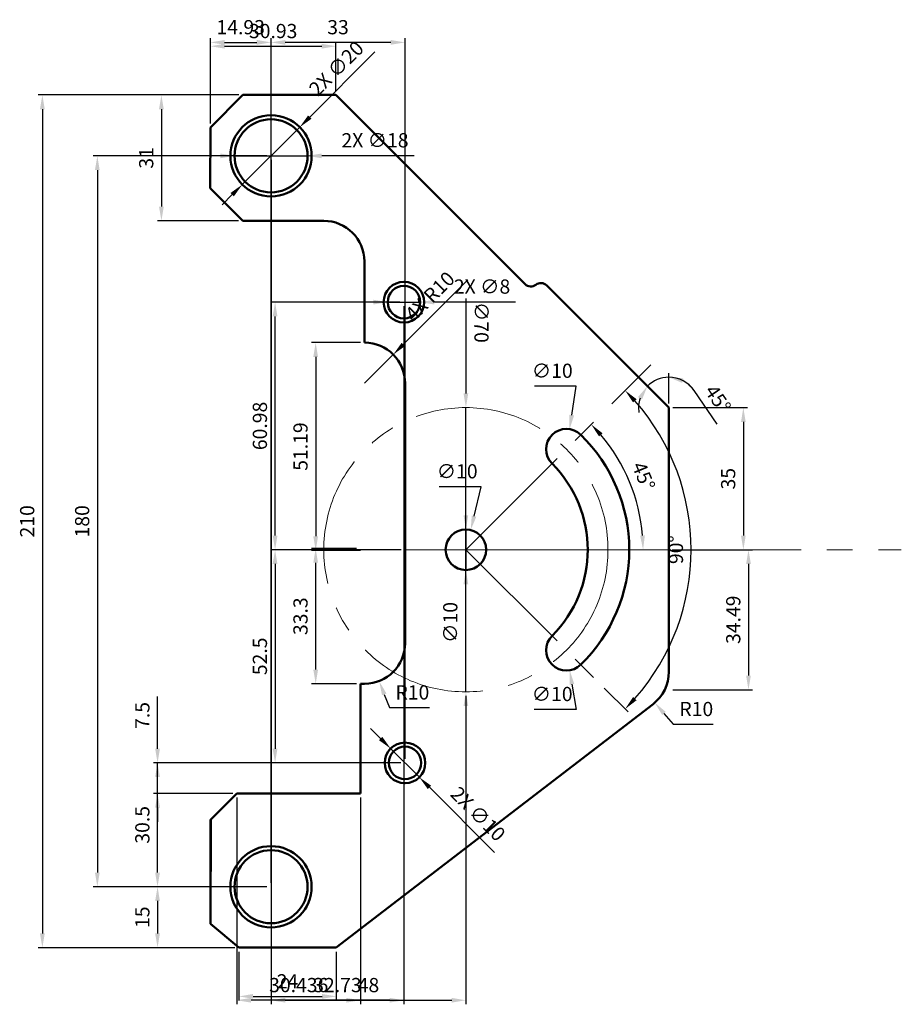
# Model space of a CAD drawing. Units: millimetres. Extents: x 1872 to 2089, y 1106 to 1349.
import ezdxf

# ---------------------------------------------------------------- set-up
doc = ezdxf.new("R2010")
doc.units = ezdxf.units.MM
doc.linetypes.add('CENTER', pattern=[50.8, 31.75, -6.35, 6.35, -6.35])
for name, color, linetype, lineweight in [('M-CNTR', 4, 'CENTER', 18), ('M-CONS', 8, 'Continuous', 13), ('M-DIMS', 3, 'Continuous', 25), ('M-OUTL', 7, 'Continuous', 50)]:
    doc.layers.add(name, color=color, linetype=linetype, lineweight=lineweight)
doc.styles.get("Standard").update_dxf_attribs({"font": 'arial.ttf'})
doc.dimstyles.new('AM_ISO$0', dxfattribs={"dimtxt": 3.5, "dimasz": 3.5, "dimexe": 1, "dimexo": 1, "dimgap": 1.5, "dimtad": 1, "dimdsep": 46, "dimtxsty": 'Standard', "dimcen": 0, "dimclrd": 256, "dimclre": 256, "dimclrt": 2, "dimadec": 0, "dimazin": 2, "dimtp": 0.1, "dimtm": 0.1, "dimtfac": 0.71, "dimtdec": 3, "dimtmove": 0, "dimatfit": 3, "dimfxl": 1, "dimlwd": -1, "dimlwe": -1, "dimarcsym": 1})
doc.dimstyles.new('AM_ISO$2', dxfattribs={"dimtxt": 3.5, "dimasz": 3.5, "dimexe": 1, "dimexo": 1, "dimgap": 1.5, "dimtad": 1, "dimdsep": 46, "dimtxsty": 'Standard', "dimcen": 0, "dimclrd": 256, "dimclre": 256, "dimclrt": 2, "dimadec": 0, "dimazin": 2, "dimtp": 0.1, "dimtm": 0.1, "dimtfac": 0.71, "dimtdec": 3, "dimtmove": 0, "dimatfit": 3, "dimfxl": 1, "dimlwd": -1, "dimlwe": -1, "dimarcsym": 1})
doc.dimstyles.new('AM_ISO$3', dxfattribs={"dimtxt": 3.5, "dimasz": 3.5, "dimexe": 1, "dimexo": 1, "dimgap": 1.5, "dimtad": 1, "dimtoh": 1, "dimdsep": 46, "dimtxsty": 'Standard', "dimcen": 0, "dimclrd": 256, "dimclre": 256, "dimclrt": 2, "dimadec": 0, "dimazin": 2, "dimtp": 0.1, "dimtm": 0.1, "dimtfac": 0.71, "dimtdec": 3, "dimtofl": 0, "dimtmove": 0, "dimatfit": 0, "dimfxl": 1, "dimlwd": -1, "dimlwe": -1, "dimarcsym": 1})
doc.dimstyles.new('AM_ISO$4', dxfattribs={"dimtxt": 3.5, "dimasz": 3.5, "dimexe": 1, "dimexo": 1, "dimgap": 1.5, "dimtad": 1, "dimtoh": 1, "dimdsep": 46, "dimtxsty": 'Standard', "dimcen": 0, "dimclrd": 256, "dimclre": 256, "dimclrt": 2, "dimadec": 0, "dimazin": 2, "dimtp": 0.1, "dimtm": 0.1, "dimtfac": 0.71, "dimtdec": 3, "dimtofl": 0, "dimtmove": 0, "dimatfit": 0, "dimfxl": 1, "dimlwd": -1, "dimlwe": -1, "dimarcsym": 1})

# ---------------------------------------------------------------- blocks, each defined once
blk = doc.blocks.new('*D3')
at = {"layer": 'Defpoints', "color": 0, "transparency": 16777216}
for p in [(2031.94, 1253.23), (2031.94, 1218.23), (2050.28, 1218.23)]:
    blk.add_point(p, dxfattribs=at)
at = {"layer": 'M-DIMS', "color": 0, "linetype": 'ByBlock', "transparency": 16777216}
for p, q in [((2032.94, 1253.23), (2051.28, 1253.23)), ((2050.28, 1249.73), (2050.28, 1221.73)), ((2032.94, 1218.23), (2051.28, 1218.23))]:
    blk.add_line(p, q, dxfattribs=at)
at = {"layer": 'M-DIMS', "color": 0, "transparency": 16777216}
for points in [[(2049.7, 1249.73), (2050.86, 1249.73), (2050.28, 1253.23)], [(2049.7, 1221.73), (2050.86, 1221.73), (2050.28, 1218.23)]]:
    blk.add_solid(points, dxfattribs=at)
at = {"layer": 'M-DIMS', "color": 0, "transparency": 16777216, "insert": (2046.99, 1235.73), "char_height": 3.5, "attachment_point": 5, "rotation": 90}
blk.add_mtext('35', dxfattribs=at)
blk = doc.blocks.new('*D4')
at = {"layer": 'Defpoints', "color": 0, "transparency": 16777216}
for p in [(2031.94, 1218.23), (2031.94, 1183.74), (2051.54, 1183.74)]:
    blk.add_point(p, dxfattribs=at)
at = {"layer": 'M-DIMS', "color": 0, "linetype": 'ByBlock', "transparency": 16777216}
for p, q in [((2032.94, 1218.23), (2052.54, 1218.23)), ((2051.54, 1214.73), (2051.54, 1187.24)), ((2032.94, 1183.74), (2052.54, 1183.74))]:
    blk.add_line(p, q, dxfattribs=at)
at = {"layer": 'M-DIMS', "color": 0, "transparency": 16777216}
for points in [[(2050.96, 1214.73), (2052.13, 1214.73), (2051.54, 1218.23)], [(2050.96, 1187.24), (2052.13, 1187.24), (2051.54, 1183.74)]]:
    blk.add_solid(points, dxfattribs=at)
at = {"layer": 'M-DIMS', "color": 0, "transparency": 16777216, "insert": (2048.25, 1200.99), "char_height": 3.5, "attachment_point": 5, "rotation": 90}
blk.add_mtext('34.49', dxfattribs=at)
blk = doc.blocks.new('*D5')
at = {"layer": 'Defpoints', "color": 0, "transparency": 16777216}
for p in [(1933.94, 1315.23), (1891.16, 1135.23), (1933.94, 1135.23)]:
    blk.add_point(p, dxfattribs=at)
at = {"layer": 'M-DIMS', "color": 0, "linetype": 'ByBlock', "transparency": 16777216}
for p, q in [((1932.94, 1315.23), (1890.16, 1315.23)), ((1891.16, 1311.73), (1891.16, 1138.73)), ((1932.94, 1135.23), (1890.16, 1135.23))]:
    blk.add_line(p, q, dxfattribs=at)
at = {"layer": 'M-DIMS', "color": 0, "transparency": 16777216}
for points in [[(1890.57, 1311.73), (1891.74, 1311.73), (1891.16, 1315.23)], [(1890.57, 1138.73), (1891.74, 1138.73), (1891.16, 1135.23)]]:
    blk.add_solid(points, dxfattribs=at)
at = {"layer": 'M-DIMS', "color": 0, "transparency": 16777216, "insert": (1887.87, 1225.23), "char_height": 3.5, "attachment_point": 5, "rotation": 90}
blk.add_mtext('180', dxfattribs=at)
blk = doc.blocks.new('*D6')
at = {"layer": 'Defpoints', "color": 0, "transparency": 16777216}
for p in [(1934.94, 1279.21), (1966.67, 1279.21), (1966.97, 1218.23)]:
    blk.add_point(p, dxfattribs=at)
at = {"layer": 'M-DIMS', "color": 0, "linetype": 'ByBlock', "transparency": 16777216}
for p, q in [((1965.67, 1279.21), (1933.94, 1279.21)), ((1934.94, 1221.73), (1934.94, 1275.71)), ((1965.97, 1218.23), (1933.94, 1218.23))]:
    blk.add_line(p, q, dxfattribs=at)
at = {"layer": 'M-DIMS', "color": 0, "transparency": 16777216}
for points in [[(1934.35, 1275.71), (1935.52, 1275.71), (1934.94, 1279.21)], [(1934.35, 1221.73), (1935.52, 1221.73), (1934.94, 1218.23)]]:
    blk.add_solid(points, dxfattribs=at)
at = {"layer": 'M-DIMS', "color": 0, "transparency": 16777216, "insert": (1931.65, 1248.72), "char_height": 3.5, "attachment_point": 5, "rotation": 90}
blk.add_mtext('60.98', dxfattribs=at)
blk = doc.blocks.new('*D7')
at = {"layer": 'Defpoints', "color": 0, "transparency": 16777216}
for p in [(1966.94, 1218.23), (1934.94, 1165.73), (1966.94, 1165.73)]:
    blk.add_point(p, dxfattribs=at)
at = {"layer": 'M-DIMS', "color": 0, "linetype": 'ByBlock', "transparency": 16777216}
for p, q in [((1965.94, 1218.23), (1933.94, 1218.23)), ((1934.94, 1214.73), (1934.94, 1169.23)), ((1965.94, 1165.73), (1933.94, 1165.73))]:
    blk.add_line(p, q, dxfattribs=at)
at = {"layer": 'M-DIMS', "color": 0, "transparency": 16777216}
for points in [[(1934.35, 1214.73), (1935.52, 1214.73), (1934.94, 1218.23)], [(1934.35, 1169.23), (1935.52, 1169.23), (1934.94, 1165.73)]]:
    blk.add_solid(points, dxfattribs=at)
at = {"layer": 'M-DIMS', "color": 0, "transparency": 16777216, "insert": (1931.65, 1191.98), "char_height": 3.5, "attachment_point": 5, "rotation": 90}
blk.add_mtext('52.5', dxfattribs=at)
blk = doc.blocks.new('*D8')
at = {"layer": 'Defpoints', "color": 0, "transparency": 16777216}
for p in [(1944.94, 1218.51), (1955.97, 1218.51), (1955.97, 1185.21)]:
    blk.add_point(p, dxfattribs=at)
at = {"layer": 'M-DIMS', "color": 0, "linetype": 'ByBlock', "transparency": 16777216}
for p, q in [((1954.97, 1218.51), (1943.94, 1218.51)), ((1944.94, 1188.71), (1944.94, 1215.01)), ((1954.97, 1185.21), (1943.94, 1185.21))]:
    blk.add_line(p, q, dxfattribs=at)
at = {"layer": 'M-DIMS', "color": 0, "transparency": 16777216}
for points in [[(1944.35, 1215.01), (1945.52, 1215.01), (1944.94, 1218.51)], [(1944.35, 1188.71), (1945.52, 1188.71), (1944.94, 1185.21)]]:
    blk.add_solid(points, dxfattribs=at)
at = {"layer": 'M-DIMS', "color": 0, "transparency": 16777216, "insert": (1941.65, 1201.86), "char_height": 3.5, "attachment_point": 5, "rotation": 90}
blk.add_mtext('33.3', dxfattribs=at)
blk = doc.blocks.new('*D9')
at = {"layer": 'Defpoints', "color": 0, "transparency": 16777216}
for p in [(1956.97, 1269.23), (1944.94, 1218.05), (1956.97, 1218.05)]:
    blk.add_point(p, dxfattribs=at)
at = {"layer": 'M-DIMS', "color": 0, "linetype": 'ByBlock', "transparency": 16777216}
for p, q in [((1955.97, 1269.23), (1943.94, 1269.23)), ((1944.94, 1265.73), (1944.94, 1221.55)), ((1955.97, 1218.05), (1943.94, 1218.05))]:
    blk.add_line(p, q, dxfattribs=at)
at = {"layer": 'M-DIMS', "color": 0, "transparency": 16777216}
for points in [[(1944.35, 1265.73), (1945.52, 1265.73), (1944.94, 1269.23)], [(1944.35, 1221.55), (1945.52, 1221.55), (1944.94, 1218.05)]]:
    blk.add_solid(points, dxfattribs=at)
at = {"layer": 'M-DIMS', "color": 0, "transparency": 16777216, "insert": (1941.65, 1243.64), "char_height": 3.5, "attachment_point": 5, "rotation": 90}
blk.add_mtext('51.19', dxfattribs=at)
blk = doc.blocks.new('*D10')
at = {"layer": 'Defpoints', "color": 0, "transparency": 16777216}
for p in [(1927.01, 1330.23), (1906.94, 1299.23), (1926.96, 1299.23)]:
    blk.add_point(p, dxfattribs=at)
at = {"layer": 'M-DIMS', "color": 0, "linetype": 'ByBlock', "transparency": 16777216}
for p, q in [((1926.01, 1330.23), (1905.94, 1330.23)), ((1906.94, 1326.73), (1906.94, 1302.73)), ((1925.96, 1299.23), (1905.94, 1299.23))]:
    blk.add_line(p, q, dxfattribs=at)
at = {"layer": 'M-DIMS', "color": 0, "transparency": 16777216}
for points in [[(1906.35, 1326.73), (1907.52, 1326.73), (1906.94, 1330.23)], [(1906.35, 1302.73), (1907.52, 1302.73), (1906.94, 1299.23)]]:
    blk.add_solid(points, dxfattribs=at)
at = {"layer": 'M-DIMS', "color": 0, "transparency": 16777216, "insert": (1903.65, 1314.73), "char_height": 3.5, "attachment_point": 5, "rotation": 90}
blk.add_mtext('31', dxfattribs=at)
blk = doc.blocks.new('*D11')
at = {"layer": 'Defpoints', "color": 0, "transparency": 16777216}
for p in [(1949.94, 1342.23), (1949.94, 1330.23), (1919.01, 1322.23)]:
    blk.add_point(p, dxfattribs=at)
at = {"layer": 'M-DIMS', "color": 0, "linetype": 'ByBlock', "transparency": 16777216}
for p, q in [((1919.01, 1323.23), (1919.01, 1343.23)), ((1922.51, 1342.23), (1946.44, 1342.23)), ((1949.94, 1331.23), (1949.94, 1343.23))]:
    blk.add_line(p, q, dxfattribs=at)
at = {"layer": 'M-DIMS', "color": 0, "transparency": 16777216}
for points in [[(1922.51, 1342.82), (1922.51, 1341.65), (1919.01, 1342.23)], [(1946.44, 1342.82), (1946.44, 1341.65), (1949.94, 1342.23)]]:
    blk.add_solid(points, dxfattribs=at)
at = {"layer": 'M-DIMS', "color": 0, "transparency": 16777216, "insert": (1934.47, 1345.52), "char_height": 3.5, "attachment_point": 5}
blk.add_mtext('30.93', dxfattribs=at)
blk = doc.blocks.new('*D12')
at = {"layer": 'Defpoints', "color": 0, "transparency": 16777216}
for p in [(1926.01, 1120.23), (1950.01, 1120.23), (1950.01, 1108.23)]:
    blk.add_point(p, dxfattribs=at)
at = {"layer": 'M-DIMS', "color": 0, "linetype": 'ByBlock', "transparency": 16777216}
for p, q in [((1926.01, 1119.23), (1926.01, 1107.23)), ((1950.01, 1119.23), (1950.01, 1107.23)), ((1929.51, 1108.23), (1946.51, 1108.23))]:
    blk.add_line(p, q, dxfattribs=at)
at = {"layer": 'M-DIMS', "color": 0, "transparency": 16777216}
for points in [[(1929.51, 1108.82), (1929.51, 1107.65), (1926.01, 1108.23)], [(1946.51, 1108.82), (1946.51, 1107.65), (1950.01, 1108.23)]]:
    blk.add_solid(points, dxfattribs=at)
at = {"layer": 'M-DIMS', "color": 0, "transparency": 16777216, "insert": (1938.01, 1111.49), "char_height": 3.5, "attachment_point": 5}
blk.add_mtext('24', dxfattribs=at)
blk = doc.blocks.new('*D13')
at = {"layer": 'Defpoints', "color": 0, "transparency": 16777216}
for p in [(1927.01, 1330.23), (1877.62, 1120.23), (1926.01, 1120.23)]:
    blk.add_point(p, dxfattribs=at)
at = {"layer": 'M-DIMS', "color": 0, "linetype": 'ByBlock', "transparency": 16777216}
for p, q in [((1926.01, 1330.23), (1876.62, 1330.23)), ((1877.62, 1326.73), (1877.62, 1123.73)), ((1925.01, 1120.23), (1876.62, 1120.23))]:
    blk.add_line(p, q, dxfattribs=at)
at = {"layer": 'M-DIMS', "color": 0, "transparency": 16777216}
for points in [[(1877.03, 1326.73), (1878.2, 1326.73), (1877.62, 1330.23)], [(1877.03, 1123.73), (1878.2, 1123.73), (1877.62, 1120.23)]]:
    blk.add_solid(points, dxfattribs=at)
at = {"layer": 'M-DIMS', "color": 0, "transparency": 16777216, "insert": (1874.33, 1225.23), "char_height": 3.5, "attachment_point": 5, "rotation": 90}
blk.add_mtext('210', dxfattribs=at)
blk = doc.blocks.new('*D14')
at = {"layer": 'Defpoints', "color": 0, "transparency": 16777216}
for p in [(2007.46, 1247.92), (2005.91, 1238.04)]:
    blk.add_point(p, dxfattribs=at)
at = {"layer": 'M-DIMS', "color": 0, "linetype": 'ByBlock', "transparency": 16777216}
for p, q in [((2009.12, 1258.48), (1998.81, 1258.48)), ((2008, 1251.38), (2009.12, 1258.48))]:
    blk.add_line(p, q, dxfattribs=at)
at = {"layer": 'M-DIMS', "color": 0, "transparency": 16777216}
blk.add_solid([(2007.43, 1251.47), (2008.58, 1251.29), (2007.46, 1247.92)], dxfattribs=at)
at = {"layer": 'M-DIMS', "color": 0, "transparency": 16777216, "insert": (2003.21, 1261.86), "char_height": 3.5, "attachment_point": 5}
blk.add_mtext('∅10', dxfattribs=at)
blk = doc.blocks.new('*D15')
at = {"layer": 'Defpoints', "color": 0, "transparency": 16777216}
for p in [(1983.12, 1223.09), (1980.76, 1213.37)]:
    blk.add_point(p, dxfattribs=at)
at = {"layer": 'M-DIMS', "color": 0, "linetype": 'ByBlock', "transparency": 16777216}
for p, q in [((1985.7, 1233.71), (1975.39, 1233.71)), ((1983.94, 1226.49), (1985.7, 1233.71))]:
    blk.add_line(p, q, dxfattribs=at)
at = {"layer": 'M-DIMS', "color": 0, "transparency": 16777216}
blk.add_solid([(1983.38, 1226.63), (1984.51, 1226.36), (1983.12, 1223.09)], dxfattribs=at)
at = {"layer": 'M-DIMS', "color": 0, "transparency": 16777216, "insert": (1979.79, 1237.1), "char_height": 3.5, "attachment_point": 5}
blk.add_mtext('∅10', dxfattribs=at)
blk = doc.blocks.new('*D16')
at = {"layer": 'Defpoints', "color": 0, "transparency": 16777216}
for p in [(2005.88, 1198.42), (2007.5, 1188.55)]:
    blk.add_point(p, dxfattribs=at)
at = {"layer": 'M-DIMS', "color": 0, "linetype": 'ByBlock', "transparency": 16777216}
for p, q in [((2008.06, 1185.1), (2009.09, 1178.87)), ((2009.09, 1178.87), (1998.78, 1178.87))]:
    blk.add_line(p, q, dxfattribs=at)
at = {"layer": 'M-DIMS', "color": 0, "transparency": 16777216}
blk.add_solid([(2008.64, 1185.19), (2007.49, 1185), (2007.5, 1188.55)], dxfattribs=at)
at = {"layer": 'M-DIMS', "color": 0, "transparency": 16777216, "insert": (2003.18, 1182.25), "char_height": 3.5, "attachment_point": 5}
blk.add_mtext('∅10', dxfattribs=at)
blk = doc.blocks.new('*D17')
at = {"layer": 'Defpoints', "color": 0, "transparency": 16777216}
for p in [(2021.94, 1188.16), (2028.45, 1180.57)]:
    blk.add_point(p, dxfattribs=at)
at = {"layer": 'M-DIMS', "color": 0, "linetype": 'ByBlock', "transparency": 16777216}
for p, q in [((2030.73, 1177.92), (2033.01, 1175.26)), ((2033.01, 1175.26), (2042.86, 1175.26))]:
    blk.add_line(p, q, dxfattribs=at)
at = {"layer": 'M-DIMS', "color": 0, "transparency": 16777216}
blk.add_solid([(2031.17, 1178.3), (2030.29, 1177.54), (2028.45, 1180.57)], dxfattribs=at)
at = {"layer": 'M-DIMS', "color": 0, "transparency": 16777216, "insert": (2038.69, 1178.55), "char_height": 3.5, "attachment_point": 5}
blk.add_mtext('R10', dxfattribs=at)
blk = doc.blocks.new('*D18')
at = {"layer": 'Defpoints', "color": 0, "transparency": 16777216}
for p in [(1956.97, 1195.21), (1960.57, 1185.88)]:
    blk.add_point(p, dxfattribs=at)
at = {"layer": 'M-DIMS', "color": 0, "linetype": 'ByBlock', "transparency": 16777216}
for p, q in [((1961.83, 1182.62), (1963.09, 1179.35)), ((1963.09, 1179.35), (1972.94, 1179.35))]:
    blk.add_line(p, q, dxfattribs=at)
at = {"layer": 'M-DIMS', "color": 0, "transparency": 16777216}
blk.add_solid([(1962.37, 1182.83), (1961.28, 1182.41), (1960.57, 1185.88)], dxfattribs=at)
at = {"layer": 'M-DIMS', "color": 0, "transparency": 16777216, "insert": (1968.76, 1182.64), "char_height": 3.5, "attachment_point": 5}
blk.add_mtext('R10', dxfattribs=at)
blk = doc.blocks.new('*D19')
at = {"layer": 'Defpoints', "color": 0, "transparency": 16777216}
for p in [(2001.83, 1283.34), (2028.2, 1259.71), (2031.94, 1253.23), (2031.94, 1253.23), (2031.94, 1188.16)]:
    blk.add_point(p, dxfattribs=at)
at = {"layer": 'M-DIMS', "color": 0, "linetype": 'ByBlock', "transparency": 16777216}
for p, q in [((2031.94, 1254.23), (2031.94, 1261.71)), ((2038.12, 1257.43), (2043.74, 1249.15))]:
    blk.add_line(p, q, dxfattribs=at)
for start, end in [(90, 135), (34.1644, 90), (35.8451, 62.9226), (162.0774, 189.1549)]:
    blk.add_arc((2031.94, 1253.23), 7.48, start, end, dxfattribs=at)
at = {"layer": 'M-DIMS', "color": 0, "transparency": 16777216}
for points in [[(2024.33, 1255.84), (2025.32, 1255.23), (2026.65, 1258.52)], [(2035.2, 1259.32), (2035.48, 1260.46), (2031.94, 1260.71)]]:
    blk.add_solid(points, dxfattribs=at)
at = {"layer": 'M-DIMS', "color": 0, "transparency": 16777216, "insert": (2043.65, 1255.13), "char_height": 3.5, "attachment_point": 5, "rotation": 304.1644}
blk.add_mtext('45°', dxfattribs=at)
blk = doc.blocks.new('*D20')
at = {"layer": 'Defpoints', "color": 0, "transparency": 16777216}
for p in [(2027.5, 1263.79), (2024.1, 1229.53), (1981.94, 1218.23), (1981.94, 1218.23), (2031.94, 1218.23)]:
    blk.add_point(p, dxfattribs=at)
at = {"layer": 'M-DIMS', "color": 0, "linetype": 'ByBlock', "transparency": 16777216}
blk.add_arc((1981.94, 1218.23), 43.64, 4.596, 40.404, dxfattribs=at)
at = {"layer": 'M-DIMS', "color": 0, "transparency": 16777216}
for points in [[(2014.74, 1246.13), (2015.6, 1246.92), (2012.8, 1249.09)], [(2026.02, 1221.75), (2024.86, 1221.71), (2025.58, 1218.23)]]:
    blk.add_solid(points, dxfattribs=at)
at = {"layer": 'M-DIMS', "color": 0, "transparency": 16777216, "insert": (2025.29, 1236.19), "char_height": 3.5, "attachment_point": 5, "rotation": 292.5}
blk.add_mtext('45°', dxfattribs=at)
blk = doc.blocks.new('*D21')
at = {"layer": 'Defpoints', "color": 0, "transparency": 16777216}
for p in [(2027.5, 1263.79), (1981.94, 1218.23), (1981.94, 1218.23), (2035.51, 1203.88), (2015.32, 1184.85)]:
    blk.add_point(p, dxfattribs=at)
at = {"layer": 'M-DIMS', "color": 0, "linetype": 'ByBlock', "transparency": 16777216}
blk.add_line((2016.03, 1184.14), (2021.87, 1178.31), dxfattribs=at)
blk.add_arc((1981.94, 1218.23), 55.47, 318.6161, 41.3839, dxfattribs=at)
at = {"layer": 'M-DIMS', "color": 0, "transparency": 16777216}
for points in [[(2023.13, 1254.5), (2023.98, 1255.3), (2021.16, 1257.45)], [(2023.98, 1181.17), (2023.13, 1181.96), (2021.16, 1179.01)]]:
    blk.add_solid(points, dxfattribs=at)
at = {"layer": 'M-DIMS', "color": 0, "transparency": 16777216, "insert": (2034.12, 1218.23), "char_height": 3.5, "attachment_point": 5, "rotation": 90}
blk.add_mtext('90°', dxfattribs=at)
blk = doc.blocks.new('LUG-HOLE-D18-CHAMFER')
for radius in [10, 9]:
    blk.add_circle((10, 10), radius)
blk = doc.blocks.new('TAPPED-HOLE-M8-CHAMFER')
for radius in [5, 4]:
    blk.add_circle((5, 5), radius)
blk = doc.blocks.new('*D24')
at = {"layer": 'Defpoints', "color": 0, "transparency": 16777216}
for p in [(1933.94, 1343.18), (1919.01, 1322.23), (1933.94, 1315.23)]:
    blk.add_point(p, dxfattribs=at)
at = {"layer": 'M-DIMS', "linetype": 'ByBlock', "transparency": 16777216}
for p, q in [((1919.01, 1323.23), (1919.01, 1344.18)), ((1933.94, 1316.23), (1933.94, 1344.18)), ((1922.51, 1343.18), (1930.44, 1343.18))]:
    blk.add_line(p, q, dxfattribs=at)
at = {"layer": 'M-DIMS', "transparency": 16777216}
for points in [[(1922.51, 1343.77), (1922.51, 1342.6), (1919.01, 1343.18)], [(1930.44, 1343.77), (1930.44, 1342.6), (1933.94, 1343.18)]]:
    blk.add_solid(points, dxfattribs=at)
at = {"layer": 'M-DIMS', "color": 2, "transparency": 16777216, "insert": (1926.47, 1346.47), "char_height": 3.5, "attachment_point": 5}
blk.add_mtext('14.93', dxfattribs=at)
blk = doc.blocks.new('*D25')
at = {"layer": 'Defpoints', "color": 0, "transparency": 16777216}
for p in [(1933.94, 1135.23), (1905.99, 1120.23), (1926.01, 1120.23)]:
    blk.add_point(p, dxfattribs=at)
at = {"layer": 'M-DIMS', "linetype": 'ByBlock', "transparency": 16777216}
for p, q in [((1932.94, 1135.23), (1904.99, 1135.23)), ((1905.99, 1131.73), (1905.99, 1123.73)), ((1925.01, 1120.23), (1904.99, 1120.23))]:
    blk.add_line(p, q, dxfattribs=at)
at = {"layer": 'M-DIMS', "transparency": 16777216}
for points in [[(1905.4, 1131.73), (1906.57, 1131.73), (1905.99, 1135.23)], [(1905.4, 1123.73), (1906.57, 1123.73), (1905.99, 1120.23)]]:
    blk.add_solid(points, dxfattribs=at)
at = {"layer": 'M-DIMS', "color": 2, "transparency": 16777216, "insert": (1902.7, 1127.73), "char_height": 3.5, "attachment_point": 5, "rotation": 90}
blk.add_mtext('15', dxfattribs=at)
blk = doc.blocks.new('*D26')
at = {"layer": 'Defpoints', "color": 0, "transparency": 16777216}
for p in [(1933.94, 1315.23), (1966.67, 1279.21), (1933.94, 1107.28)]:
    blk.add_point(p, dxfattribs=at)
at = {"layer": 'M-DIMS', "linetype": 'ByBlock', "transparency": 16777216}
for p, q in [((1933.94, 1314.23), (1933.94, 1106.28)), ((1966.67, 1278.21), (1966.67, 1106.28)), ((1963.17, 1107.28), (1937.44, 1107.28))]:
    blk.add_line(p, q, dxfattribs=at)
at = {"layer": 'M-DIMS', "transparency": 16777216}
for points in [[(1937.44, 1107.87), (1937.44, 1106.7), (1933.94, 1107.28)], [(1963.17, 1107.87), (1963.17, 1106.7), (1966.67, 1107.28)]]:
    blk.add_solid(points, dxfattribs=at)
at = {"layer": 'M-DIMS', "color": 2, "transparency": 16777216, "insert": (1950.3, 1110.57), "char_height": 3.5, "attachment_point": 5}
blk.add_mtext('32.73', dxfattribs=at)
blk = doc.blocks.new('*D27')
at = {"layer": 'Defpoints', "color": 0, "transparency": 16777216}
for p in [(1933.94, 1343.18), (1966.94, 1165.73), (1933.94, 1135.23)]:
    blk.add_point(p, dxfattribs=at)
at = {"layer": 'M-DIMS', "linetype": 'ByBlock', "transparency": 16777216}
for p, q in [((1933.94, 1136.23), (1933.94, 1344.18)), ((1966.94, 1166.73), (1966.94, 1344.18)), ((1963.44, 1343.18), (1937.44, 1343.18))]:
    blk.add_line(p, q, dxfattribs=at)
at = {"layer": 'M-DIMS', "transparency": 16777216}
for points in [[(1937.44, 1343.77), (1937.44, 1342.6), (1933.94, 1343.18)], [(1963.44, 1343.77), (1963.44, 1342.6), (1966.94, 1343.18)]]:
    blk.add_solid(points, dxfattribs=at)
at = {"layer": 'M-DIMS', "color": 2, "transparency": 16777216, "insert": (1950.44, 1346.47), "char_height": 3.5, "attachment_point": 5}
blk.add_mtext('33', dxfattribs=at)
blk = doc.blocks.new('*D28')
at = {"layer": 'Defpoints', "color": 0, "transparency": 16777216}
for p in [(1981.94, 1183.23), (1933.94, 1135.23), (1981.94, 1107.28)]:
    blk.add_point(p, dxfattribs=at)
at = {"layer": 'M-DIMS', "linetype": 'ByBlock', "transparency": 16777216}
for p, q in [((1981.94, 1182.23), (1981.94, 1106.28)), ((1933.94, 1134.23), (1933.94, 1106.28)), ((1937.44, 1107.28), (1978.44, 1107.28))]:
    blk.add_line(p, q, dxfattribs=at)
at = {"layer": 'M-DIMS', "transparency": 16777216}
for points in [[(1937.44, 1107.87), (1937.44, 1106.7), (1933.94, 1107.28)], [(1978.44, 1107.87), (1978.44, 1106.7), (1981.94, 1107.28)]]:
    blk.add_solid(points, dxfattribs=at)
at = {"layer": 'M-DIMS', "color": 2, "transparency": 16777216, "insert": (1957.94, 1110.57), "char_height": 3.5, "attachment_point": 5}
blk.add_mtext('48', dxfattribs=at)
blk = doc.blocks.new('*D29')
at = {"layer": 'Defpoints', "color": 0, "transparency": 16777216}
for p in [(1905.99, 1165.73), (1966.94, 1165.73), (1933.94, 1135.23)]:
    blk.add_point(p, dxfattribs=at)
at = {"layer": 'M-DIMS', "linetype": 'ByBlock', "transparency": 16777216}
for p, q in [((1965.94, 1165.73), (1904.99, 1165.73)), ((1905.99, 1138.73), (1905.99, 1162.23)), ((1932.94, 1135.23), (1904.99, 1135.23))]:
    blk.add_line(p, q, dxfattribs=at)
at = {"layer": 'M-DIMS', "transparency": 16777216}
for points in [[(1905.4, 1162.23), (1906.57, 1162.23), (1905.99, 1165.73)], [(1905.4, 1138.73), (1906.57, 1138.73), (1905.99, 1135.23)]]:
    blk.add_solid(points, dxfattribs=at)
at = {"layer": 'M-DIMS', "color": 2, "transparency": 16777216, "insert": (1902.7, 1150.48), "char_height": 3.5, "attachment_point": 5, "rotation": 90}
blk.add_mtext('30.5', dxfattribs=at)
blk = doc.blocks.new('*D30')
at = {"layer": 'Defpoints', "color": 0, "transparency": 16777216}
for p in [(1925.54, 1158.23), (1955.97, 1158.23), (1925.54, 1107.28)]:
    blk.add_point(p, dxfattribs=at)
at = {"layer": 'M-DIMS', "linetype": 'ByBlock', "transparency": 16777216}
for p, q in [((1925.54, 1157.23), (1925.54, 1106.28)), ((1955.97, 1157.23), (1955.97, 1106.28)), ((1952.47, 1107.28), (1929.04, 1107.28))]:
    blk.add_line(p, q, dxfattribs=at)
at = {"layer": 'M-DIMS', "transparency": 16777216}
for points in [[(1929.04, 1107.87), (1929.04, 1106.7), (1925.54, 1107.28)], [(1952.47, 1107.87), (1952.47, 1106.7), (1955.97, 1107.28)]]:
    blk.add_solid(points, dxfattribs=at)
at = {"layer": 'M-DIMS', "color": 2, "transparency": 16777216, "insert": (1940.76, 1110.57), "char_height": 3.5, "attachment_point": 5}
blk.add_mtext('30.436', dxfattribs=at)
blk = doc.blocks.new('*D31')
at = {"layer": 'Defpoints', "color": 0, "transparency": 16777216}
for p in [(1905.99, 1165.73), (1966.94, 1165.73), (1925.54, 1158.23)]:
    blk.add_point(p, dxfattribs=at)
at = {"layer": 'M-DIMS', "linetype": 'ByBlock', "transparency": 16777216}
for p, q in [((1905.99, 1169.23), (1905.99, 1182.1)), ((1965.94, 1165.73), (1904.99, 1165.73)), ((1905.99, 1158.23), (1905.99, 1165.73)), ((1924.54, 1158.23), (1904.99, 1158.23)), ((1905.99, 1154.73), (1905.99, 1151.23))]:
    blk.add_line(p, q, dxfattribs=at)
at = {"layer": 'M-DIMS', "transparency": 16777216}
for points in [[(1905.4, 1169.23), (1906.57, 1169.23), (1905.99, 1165.73)], [(1905.4, 1154.73), (1906.57, 1154.73), (1905.99, 1158.23)]]:
    blk.add_solid(points, dxfattribs=at)
at = {"layer": 'M-DIMS', "color": 2, "transparency": 16777216, "insert": (1902.71, 1177.42), "char_height": 3.5, "attachment_point": 5, "rotation": 90}
blk.add_mtext('7.5', dxfattribs=at)
blk = doc.blocks.new('*D32')
at = {"layer": 'Defpoints', "color": 0, "transparency": 16777216}
for p in [(1924.94, 1315.23), (1942.94, 1315.23)]:
    blk.add_point(p, dxfattribs=at)
at = {"layer": 'M-DIMS', "linetype": 'ByBlock', "transparency": 16777216}
for p, q in [((1921.44, 1315.23), (1917.94, 1315.23)), ((1924.94, 1315.23), (1942.94, 1315.23)), ((1969.16, 1315.24), (1946.44, 1315.23))]:
    blk.add_line(p, q, dxfattribs=at)
at = {"layer": 'M-DIMS', "transparency": 16777216}
for points in [[(1921.44, 1315.82), (1921.44, 1314.65), (1924.94, 1315.23)], [(1946.44, 1315.82), (1946.44, 1314.65), (1942.94, 1315.23)]]:
    blk.add_solid(points, dxfattribs=at)
at = {"layer": 'M-DIMS', "color": 2, "transparency": 16777216, "insert": (1959.55, 1318.62), "char_height": 3.5, "attachment_point": 5, "rotation": 0.0023}
blk.add_mtext('2X ∅18', dxfattribs=at)
blk = doc.blocks.new('*D33')
at = {"layer": 'Defpoints', "color": 0, "transparency": 16777216}
for p in [(1941.01, 1322.3), (1926.87, 1308.16)]:
    blk.add_point(p, dxfattribs=at)
at = {"layer": 'M-DIMS', "linetype": 'ByBlock', "transparency": 16777216}
for p, q in [((1959.54, 1340.83), (1943.48, 1324.78)), ((1926.87, 1308.16), (1941.01, 1322.3)), ((1924.39, 1305.69), (1921.92, 1303.21))]:
    blk.add_line(p, q, dxfattribs=at)
at = {"layer": 'M-DIMS', "transparency": 16777216}
for points in [[(1943.07, 1325.19), (1943.9, 1324.37), (1941.01, 1322.3)], [(1923.98, 1306.1), (1924.8, 1305.28), (1926.87, 1308.16)]]:
    blk.add_solid(points, dxfattribs=at)
at = {"layer": 'M-DIMS', "color": 2, "transparency": 16777216, "insert": (1950.36, 1336.44), "char_height": 3.5, "attachment_point": 5, "rotation": 44.9985}
blk.add_mtext('2X ∅20', dxfattribs=at)
blk = doc.blocks.new('*D34')
at = {"layer": 'Defpoints', "color": 0, "transparency": 16777216}
for p in [(1962.67, 1279.21), (1970.67, 1279.21)]:
    blk.add_point(p, dxfattribs=at)
at = {"layer": 'M-DIMS', "linetype": 'ByBlock', "transparency": 16777216}
for p, q in [((1959.17, 1279.21), (1955.67, 1279.21)), ((1962.67, 1279.21), (1970.67, 1279.21)), ((1994.17, 1279.21), (1974.17, 1279.21))]:
    blk.add_line(p, q, dxfattribs=at)
at = {"layer": 'M-DIMS', "transparency": 16777216}
for points in [[(1959.17, 1279.8), (1959.17, 1278.63), (1962.67, 1279.21)], [(1974.17, 1279.79), (1974.17, 1278.63), (1970.67, 1279.21)]]:
    blk.add_solid(points, dxfattribs=at)
at = {"layer": 'M-DIMS', "color": 2, "transparency": 16777216, "insert": (1985.92, 1282.59), "char_height": 3.5, "attachment_point": 5, "rotation": 359.993}
blk.add_mtext('2X ∅8', dxfattribs=at)
blk = doc.blocks.new('*D35')
at = {"layer": 'Defpoints', "color": 0, "transparency": 16777216}
for p in [(1963.4, 1169.27), (1970.47, 1162.2)]:
    blk.add_point(p, dxfattribs=at)
at = {"layer": 'M-DIMS', "linetype": 'ByBlock', "transparency": 16777216}
for p, q in [((1960.93, 1171.74), (1958.45, 1174.22)), ((1963.4, 1169.27), (1970.47, 1162.2)), ((1989, 1143.67), (1972.95, 1159.72))]:
    blk.add_line(p, q, dxfattribs=at)
at = {"layer": 'M-DIMS', "transparency": 16777216}
for points in [[(1961.34, 1172.16), (1960.52, 1171.33), (1963.4, 1169.27)], [(1973.36, 1160.14), (1972.54, 1159.31), (1970.47, 1162.2)]]:
    blk.add_solid(points, dxfattribs=at)
at = {"layer": 'M-DIMS', "color": 2, "transparency": 16777216, "insert": (1984.61, 1152.85), "char_height": 3.5, "attachment_point": 5, "rotation": 315.0007}
blk.add_mtext('2X ∅10', dxfattribs=at)
blk = doc.blocks.new('*D36')
at = {"layer": 'Defpoints', "color": 0, "transparency": 16777216}
for p in [(1981.94, 1223.23), (1981.94, 1213.23)]:
    blk.add_point(p, dxfattribs=at)
at = {"layer": 'M-DIMS', "linetype": 'ByBlock', "transparency": 16777216}
for p, q in [((1981.94, 1226.73), (1981.94, 1230.23)), ((1981.94, 1223.23), (1981.94, 1213.23)), ((1981.94, 1194.42), (1981.94, 1209.73))]:
    blk.add_line(p, q, dxfattribs=at)
at = {"layer": 'M-DIMS', "transparency": 16777216}
for points in [[(1981.36, 1226.73), (1982.52, 1226.73), (1981.94, 1223.23)], [(1981.35, 1209.73), (1982.52, 1209.73), (1981.94, 1213.23)]]:
    blk.add_solid(points, dxfattribs=at)
at = {"layer": 'M-DIMS', "color": 2, "transparency": 16777216, "insert": (1978.55, 1200.33), "char_height": 3.5, "attachment_point": 5, "rotation": 89.9968}
blk.add_mtext('∅10', dxfattribs=at)
blk = doc.blocks.new('*D37')
at = {"layer": 'Defpoints', "color": 0, "transparency": 16777216}
for p in [(1981.94, 1253.23), (1981.94, 1183.23)]:
    blk.add_point(p, dxfattribs=at)
at = {"layer": 'M-DIMS', "linetype": 'ByBlock', "transparency": 16777216}
for p, q in [((1981.94, 1280.14), (1981.94, 1256.73)), ((1981.94, 1183.23), (1981.94, 1253.23)), ((1981.94, 1179.73), (1981.94, 1176.23))]:
    blk.add_line(p, q, dxfattribs=at)
at = {"layer": 'M-DIMS', "transparency": 16777216}
for points in [[(1982.52, 1256.73), (1981.35, 1256.73), (1981.94, 1253.23)], [(1982.52, 1179.73), (1981.36, 1179.73), (1981.94, 1183.23)]]:
    blk.add_solid(points, dxfattribs=at)
at = {"layer": 'M-DIMS', "color": 2, "transparency": 16777216, "insert": (1985.32, 1274.23), "char_height": 3.5, "attachment_point": 5, "rotation": 270.0005}
blk.add_mtext('∅70', dxfattribs=at)
blk = doc.blocks.new('*D38')
at = {"layer": 'Defpoints', "color": 0, "transparency": 16777216}
for p in [(1964.04, 1266.3), (1956.97, 1259.23)]:
    blk.add_point(p, dxfattribs=at)
at = {"layer": 'M-DIMS', "linetype": 'ByBlock', "transparency": 16777216}
for p, q in [((1982.44, 1284.7), (1966.52, 1268.78)), ((1956.97, 1259.23), (1964.04, 1266.3))]:
    blk.add_line(p, q, dxfattribs=at)
at = {"layer": 'M-DIMS', "transparency": 16777216}
blk.add_solid([(1966.11, 1269.19), (1966.93, 1268.37), (1964.04, 1266.3)], dxfattribs=at)
at = {"layer": 'M-DIMS', "color": 2, "transparency": 16777216, "insert": (1973.39, 1280.3), "char_height": 3.5, "attachment_point": 5, "rotation": 45.0018}
blk.add_mtext('4X R10', dxfattribs=at)

msp = doc.modelspace()

# ---------------------------------------------------------------- linework, layer by layer
at = {"layer": 'M-CNTR'}
for q in [(2027.4986, 1263.794), (2089.1852, 1218.2336), (2015.3205, 1184.8514)]:
    msp.add_line((1981.9383, 1218.2336), q, dxfattribs=at)
msp.add_circle((1981.9383, 1218.2336), 35, dxfattribs=at)
at = {"layer": 'M-CONS'}
for p, q in [((1942.9383, 1315.2336), (1943.9383, 1315.2336)), ((1981.9383, 1223.2336), (1981.9383, 1218.2336)), ((1981.9383, 1218.2336), (1966.9383, 1218.2336)), ((1981.9383, 1218.2336), (1976.9383, 1218.2336)), ((1981.9383, 1218.2336), (2031.9383, 1218.2336))]:
    msp.add_line(p, q, dxfattribs=at)
at = {"layer": 'M-OUTL'}
for p, q in [((1919.0069, 1322.2339), (1927.0066, 1330.2336)), ((1927.0066, 1330.2336), (1933.9383, 1330.2336)), ((1927.0066, 1330.2336), (1949.9383, 1330.2336)), ((1949.9383, 1330.2336), (1996.5241, 1283.6479)), ((1919.0069, 1322.2339), (1918.9383, 1307.2523)), ((1926.9569, 1299.2336), (1918.9383, 1307.2523)), ((1926.9569, 1299.2336), (1946.9383, 1299.2336)), ((1956.9383, 1269.2336), (1956.9383, 1289.2336)), ((2031.9383, 1253.2336), (2001.8334, 1283.3386)), ((1956.9383, 1269.2336), (1956.9731, 1269.2336)), ((1966.9731, 1217.2122), (1966.9731, 1259.2336)), ((2031.9383, 1188.1588), (2031.9383, 1253.2336)), ((2031.9383, 1218.2336), (2031.9383, 1188.1588)), ((1966.9731, 1217.2122), (1966.9731, 1195.2122)), ((1956.9731, 1185.2122), (1955.9731, 1185.2122)), ((1955.9731, 1185.2122), (1955.9731, 1158.2335)), ((1950.0066, 1120.2336), (2028.0339, 1180.2314)), ((1925.5375, 1158.2335), (1919.0066, 1151.7025)), ((1925.5375, 1158.2335), (1955.9731, 1158.2335)), ((1919.0066, 1151.7025), (1919.0066, 1126.077)), ((1919.0218, 1126.0642), (1919.0892, 1151.7852)), ((1926.0066, 1120.2336), (1919.0066, 1126.077)), ((1950.0066, 1120.2336), (1926.0066, 1120.2336))]:
    msp.add_line(p, q, dxfattribs=at)
msp.add_circle((1981.9383, 1218.2336), 5, dxfattribs=at)
for centre, radius, start, end in [((1946.9383, 1289.2336), 10, 0, 90), ((1997.9383, 1285.0621), 2, 225, 308.331971), ((2000.4191, 1281.9243), 2, 45, 128.331971), ((1956.9731, 1259.2336), 10, 0, 90), ((2006.687, 1242.9824), 5, 45, 225), ((1982.7117, 1218.2336), 39.4569, 314.205868, 45.794132), ((1981.9383, 1218.2336), 30, 315, 45), ((2006.687, 1193.4849), 5, 135, 315), ((1956.9731, 1195.2122), 10, 270, 0), ((2021.9383, 1188.1588), 10, 307.557872, 0)]:
    msp.add_arc(centre, radius, start, end, dxfattribs=at)

# ---------------------------------------------------------------- block references
for name, p in [('LUG-HOLE-D18-CHAMFER', (1923.938, 1305.234)), ('TAPPED-HOLE-M8-CHAMFER', (1961.6707, 1274.2118)), ('TAPPED-HOLE-M8-CHAMFER', (1961.938, 1160.734)), ('LUG-HOLE-D18-CHAMFER', (1923.938, 1125.234))]:
    msp.add_blockref(name, p, dxfattribs=at)

# ---------------------------------------------------------------- dimensions: what is measured, and where the dimension line sits
at = {"layer": 'M-DIMS'}
for base, p1, p2, override, picture, middle in [((1933.9383, 1343.1836), (1919.0069, 1322.2339), (1933.9383, 1315.2336), {"dimdec": 2, "dimlfac": 1, "dimrnd": 0, "dimzin": 0, "dimdsep": 46, "dimlunit": 2}, '*D24', (1926.4726, 1346.4718)), ((1933.9383, 1343.1836), (1966.9383, 1165.7336), (1933.9383, 1135.2336), {"dimdec": 0, "dimlfac": 1, "dimrnd": 0, "dimzin": 0, "dimdsep": 46, "dimlunit": 2}, '*D27', (1950.4383, 1346.4718)), ((1949.9383, 1342.2336), (1919.0069, 1322.2339), (1949.9383, 1330.2336), {"dimpost": '', "dimclrd": 0, "dimclre": 0, "dimclrt": 0}, '*D11', (1934.4726, 1345.5218)), ((1933.9383, 1107.2836), (1966.671, 1279.2115), (1933.9383, 1315.2336), {"dimdec": 2, "dimlfac": 1, "dimrnd": 0, "dimzin": 0, "dimdsep": 46, "dimlunit": 2}, '*D26', (1950.3046, 1110.5718)), ((1981.9383, 1107.2836), (1933.9383, 1135.2336), (1981.9383, 1183.2336), {"dimdec": 0, "dimlfac": 1, "dimrnd": 0, "dimzin": 0, "dimdsep": 46, "dimlunit": 2}, '*D28', (1957.9383, 1110.5706)), ((1925.5375, 1107.2836), (1955.9731, 1158.2335), (1925.5375, 1158.2335), {"dimdec": 3, "dimlfac": 1, "dimrnd": 0, "dimzin": 0, "dimdsep": 46, "dimlunit": 2}, '*D30', (1940.7553, 1110.5718))]:
    dim = msp.add_linear_dim(base=base, p1=p1, p2=p2, dimstyle='AM_ISO$0', override=override, dxfattribs=at)
    dim.commit()
    dim.dimension.update_dxf_attribs({"geometry": picture, "text_midpoint": middle})
for p1, p2, picture, middle in [((1926.867, 1308.1628), (1941.0095, 1322.3045), '*D33', (1952.7491, 1334.0435)), ((1924.9383, 1315.2333), (1942.9383, 1315.234), '*D32', (1959.5496, 1315.2347))]:
    dim = msp.add_diameter_dim_2p(p1=p1, p2=p2, text='2X <>', dimstyle='AM_ISO$0', override={"dimdec": 0, "dimlfac": 1, "dimrnd": 0, "dimzin": 0, "dimdsep": 46, "dimlunit": 2}, dxfattribs=at)
    dim.commit()
    dim.dimension.update_dxf_attribs({"geometry": picture, "text_midpoint": middle, "dimtype": 163})
for base, p1, p2, angle, override, picture, middle in [((1877.6167, 1120.2336), (1927.0066, 1330.2336), (1926.0066, 1120.2336), 90, {"dimpost": '', "dimclrd": 0, "dimclre": 0, "dimclrt": 0}, '*D13', (1874.3297, 1225.2336)), ((1906.9383, 1299.2336), (1927.0066, 1330.2336), (1926.9569, 1299.2336), 90, {"dimpost": '', "dimclrd": 0, "dimclre": 0, "dimclrt": 0}, '*D10', (1903.6501, 1314.7336)), ((1891.1558, 1135.2336), (1933.9383, 1315.2336), (1933.9383, 1135.2336), 90, {"dimpost": '', "dimclrd": 0, "dimclre": 0, "dimclrt": 0}, '*D5', (1887.8688, 1225.2336)), ((1934.9383, 1279.2115), (1966.9731, 1218.2336), (1966.671, 1279.2115), 90, {"dimpost": '', "dimclrd": 0, "dimclre": 0, "dimclrt": 0}, '*D6', (1931.6513, 1248.7226)), ((1944.9383, 1218.0468), (1956.9731, 1269.2336), (1956.9731, 1218.0468), 90, {"dimpost": '', "dimclrd": 0, "dimclre": 0, "dimclrt": 0}, '*D9', (1941.6513, 1243.6402)), ((2050.2799, 1218.2336), (2031.9383, 1253.2336), (2031.9383, 1218.2336), 90, {"dimpost": '', "dimclrd": 0, "dimclre": 0, "dimclrt": 0}, '*D3', (2046.9917, 1235.7336)), ((1934.9383, 1165.7336), (1966.9383, 1218.2336), (1966.9383, 1165.7336), 90, {"dimpost": '', "dimclrd": 0, "dimclre": 0, "dimclrt": 0}, '*D7', (1931.6513, 1191.9836)), ((1944.9383, 1218.5142), (1955.9731, 1185.2122), (1955.9731, 1218.5142), 90, {"dimpost": '', "dimclrd": 0, "dimclre": 0, "dimclrt": 0}, '*D8', (1941.6501, 1201.8632)), ((2051.543, 1183.7405), (2031.9383, 1218.2336), (2031.9383, 1183.7405), 90, {"dimpost": '', "dimclrd": 0, "dimclre": 0, "dimclrt": 0}, '*D4', (2048.2548, 1200.9871)), ((1905.9883, 1165.7336), (1925.5375, 1158.2335), (1966.9383, 1165.7336), 90, {"dimdec": 1, "dimlfac": 1, "dimrnd": 0, "dimzin": 0, "dimdsep": 46, "dimlunit": 2}, '*D31', (1902.7084, 1177.4185)), ((1905.9883, 1165.7336), (1933.9383, 1135.2336), (1966.9383, 1165.7336), 90, {"dimdec": 1, "dimlfac": 1, "dimrnd": 0, "dimzin": 0, "dimdsep": 46, "dimlunit": 2}, '*D29', (1902.7001, 1150.4836)), ((1905.9883, 1120.2336), (1933.9383, 1135.2336), (1926.0066, 1120.2336), 90, {"dimdec": 0, "dimlfac": 1, "dimrnd": 0, "dimzin": 0, "dimdsep": 46, "dimlunit": 2}, '*D25', (1902.7013, 1127.7336)), ((1950.0066, 1108.2336), (1926.0066, 1120.2336), (1950.0066, 1120.2336), 0, {"dimpost": '', "dimclrd": 0, "dimclre": 0, "dimclrt": 0}, '*D12', (1938.0066, 1111.4908))]:
    dim = msp.add_linear_dim(base=base, p1=p1, p2=p2, angle=angle, dimstyle='AM_ISO$0', override=override, dxfattribs=at)
    dim.commit()
    dim.dimension.update_dxf_attribs({"geometry": picture, "text_midpoint": middle})
for p1, p2, picture, middle in [((1962.671, 1279.212), (1970.671, 1279.211), '*D34', (1985.9227, 1279.2091)), ((1963.4027, 1169.2691), (1970.4739, 1162.1981), '*D35', (1982.2132, 1150.459))]:
    dim = msp.add_diameter_dim_2p(p1=p1, p2=p2, text='2X <>', dimstyle='AM_ISO$0', override={"dimdec": 0, "dimlfac": 1, "dimrnd": 0, "dimzin": 0, "dimdsep": 46, "dimlunit": 2}, dxfattribs=at)
    dim.commit()
    dim.dimension.update_dxf_attribs({"geometry": picture, "text_midpoint": middle})
dim = msp.add_radius_dim(center=(1956.9731, 1259.2336), mpoint=(1964.0439, 1266.3049), text='4X <>', dimstyle='AM_ISO$0', override={"dimdec": 0, "dimlfac": 1, "dimrnd": 0, "dimzin": 0, "dimdsep": 46, "dimlunit": 2}, dxfattribs=at)
dim.commit()
dim.dimension.update_dxf_attribs({"geometry": '*D38', "text_midpoint": (1973.3909, 1280.3012)})
for base, line1, line2, override, picture, middle in [((2028.2006, 1259.7075), ((2031.9383, 1253.2336), (2001.8334, 1283.3386)), ((2031.9383, 1188.1588), (2031.9383, 1253.2336)), {"dimpost": '', "dimclrd": 0, "dimclre": 0, "dimclrt": 0}, '*D19', (2043.6473, 1255.1333)), ((2024.0951, 1229.5295), ((1981.9383, 1218.2336), (2031.9383, 1218.2336)), ((1981.9383, 1218.2336), (2027.4986, 1263.794)), {"dimpost": '', "dimclrd": 0, "dimclre": 0, "dimclrt": 0}, '*D20', (2025.2902, 1236.1906)), ((2035.5135, 1203.8782), ((1981.9383, 1218.2336), (2027.4986, 1263.794)), ((1981.9383, 1218.2336), (2015.3205, 1184.8514)), {"dimclrd": 0, "dimclre": 0, "dimclrt": 0}, '*D21', (2034.1164, 1218.2336))]:
    dim = msp.add_angular_dim_2l(base=base, line1=line1, line2=line2, dimstyle='AM_ISO$2', override=override, dxfattribs=at)
    dim.commit()
    dim.dimension.update_dxf_attribs({"geometry": picture, "text_midpoint": middle})
for p1, p2, dimstyle, override, picture, middle in [((1981.9385, 1183.2336), (1981.938, 1253.2336), 'AM_ISO$0', {"dimdec": 0, "dimlfac": 1, "dimrnd": 0, "dimzin": 0, "dimdsep": 46, "dimlunit": 2}, '*D37', (1981.9378, 1274.2336)), ((2005.9128, 1238.0427), (2007.4612, 1247.9221), 'AM_ISO$3', {"dimpost": '', "dimclrd": 0, "dimclre": 0, "dimclrt": 0}, '*D14', (2003.2112, 1258.4798)), ((1980.7588, 1213.3747), (1983.1177, 1223.0925), 'AM_ISO$3', {"dimclrd": 0, "dimclre": 0, "dimclrt": 0}, '*D15', (1979.7912, 1233.7143)), ((2005.8765, 1198.4188), (2007.4975, 1188.551), 'AM_ISO$3', {"dimclrd": 0, "dimclre": 0, "dimclrt": 0}, '*D16', (2003.1838, 1178.8651))]:
    dim = msp.add_diameter_dim_2p(p1=p1, p2=p2, dimstyle=dimstyle, override=override, dxfattribs=at)
    dim.commit()
    dim.dimension.update_dxf_attribs({"geometry": picture, "text_midpoint": middle, "dimtype": 163})
dim = msp.add_diameter_dim_2p(p1=(1981.9385, 1223.2336), p2=(1981.938, 1213.2336), dimstyle='AM_ISO$0', override={"dimdec": 0, "dimlfac": 1, "dimrnd": 0, "dimzin": 0, "dimdsep": 46, "dimlunit": 2}, dxfattribs=at)
dim.commit()
dim.dimension.update_dxf_attribs({"geometry": '*D36', "text_midpoint": (1981.9373, 1200.3288)})
for center, mpoint, override, picture, middle in [((1956.9731, 1195.2122), (1960.5691, 1185.8812), {"dimclrd": 0, "dimclre": 0, "dimclrt": 0}, '*D18', (1968.7619, 1179.3494)), ((2021.9383, 1188.1588), (2028.452, 1180.5712), {"dimpost": '', "dimclrd": 0, "dimclre": 0, "dimclrt": 0}, '*D17', (2038.6872, 1175.2599))]:
    dim = msp.add_radius_dim(center=center, mpoint=mpoint, dimstyle='AM_ISO$4', override=override, dxfattribs=at)
    dim.commit()
    dim.dimension.update_dxf_attribs({"geometry": picture, "text_midpoint": middle, "dimtype": 164})

doc.saveas('drawing.dxf')
